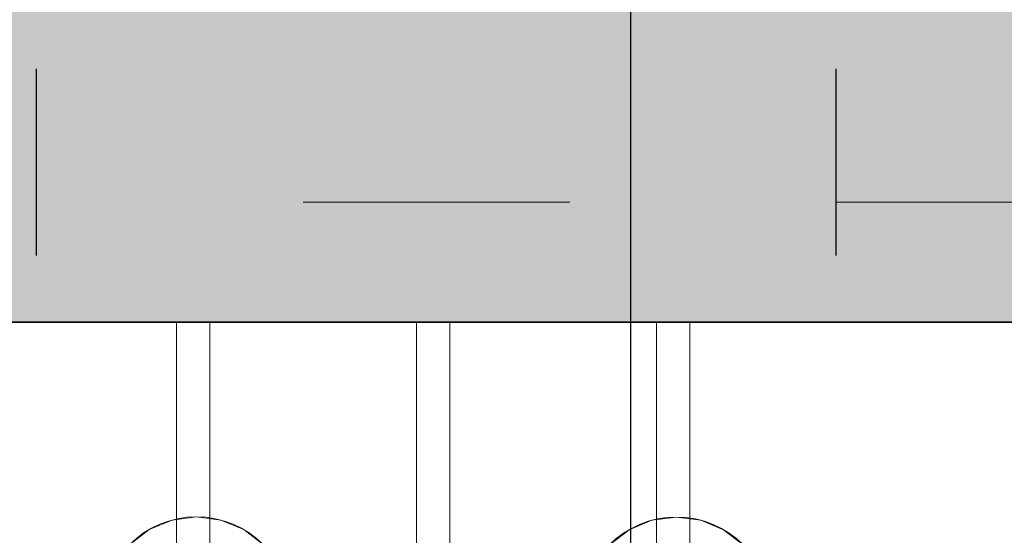
# Model space of a CAD drawing. Units: inches. Extents: x 2696 to 3240, y 1564 to 2310.
# Tile 46 of 76: x 2777.108 to 2786.339, y 2089.203 to 2094.037. Entities that reach past the tile are written whole.
import ezdxf

# ---------------------------------------------------------------- set-up
doc = ezdxf.new("R2010")
doc.units = ezdxf.units.IN
for name, color, linetype, lineweight in [('A-ANNO-DIMS', 3, 'Continuous', 18), ('A-FLOR-FIXT', 8, 'Continuous', 18), ('A-FURN', 251, 'Continuous', 13), ('A-WALL', 7, 'Continuous', 35), ('A-WALL-PATT', 9, 'Continuous', 13)]:
    doc.layers.add(name, color=color, linetype=linetype, lineweight=lineweight)
doc.layers.add('FURNITURE', color=250, linetype='Continuous')
doc.styles.add('TIMES NEW', font='times.ttf')
doc.dimstyles.new('Siddhuu', dxfattribs={"dimtxt": 6, "dimasz": 2.5, "dimexe": 1.25, "dimexo": 0.625, "dimtad": 1, "dimdec": 1, "dimlunit": 4, "dimtxsty": 'TIMES NEW', "dimcen": 2.5, "dimclrd": 256, "dimclre": 1, "dimclrt": 7, "dimadec": 0, "dimazin": 0, "dimtfac": 1, "dimtdec": 1, "dimtmove": 0, "dimatfit": 3, "dimfxl": 1, "dimtolj": 1, "dimlwd": -1, "dimarcsym": 0})

# ---------------------------------------------------------------- blocks, each defined once
blk = doc.blocks.new('A$C1af1f523')
at = {"layer": 'A-FURN'}
for p, q in [((-1.9455, 2.8785), (-1.9455, 2.8785, 0.5)), ((-1.857, 2.6648), (-1.857, 2.6648, 0.5)), ((0, 2.5605), (-4.2116, 2.5605)), ((0, 2.5605, 0.5), (-4.2116, 2.5605, 0.5)), ((-1.8268, 2.4355), (-1.8268, 2.4355, 0.5)), ((0, 2.248), (-4.2116, 2.248)), ((0, 2.248, 0.5), (-4.2116, 2.248, 0.5)), ((-1.857, 2.2061), (-1.857, 2.2061, 0.5)), ((-1.9455, 1.9924), (-1.9455, 1.9924, 0.5)), ((0, 0.3125), (-6.5015, 0.3125)), ((0, 0.3125, 0.5), (-6.5015, 0.3125, 0.5)), ((0, 0), (-6.5015, 0)), ((0, 0, 0.5), (-6.5015, 0, 0.5)), ((-1.9432, -1.6208), (-1.9432, -1.6208, 0.5)), ((-1.8547, -1.8345), (-1.8547, -1.8345, 0.5)), ((0, -1.9388), (-4.2094, -1.9388)), ((0, -1.9388, 0.5), (-4.2094, -1.9388, 0.5)), ((-1.8245, -2.0638), (-1.8245, -2.0638, 0.5)), ((0, -2.2513), (-4.2094, -2.2513)), ((0, -2.2513, 0.5), (-4.2094, -2.2513, 0.5)), ((-1.8547, -2.2931), (-1.8547, -2.2931, 0.5)), ((-1.9432, -2.5068), (-1.9432, -2.5068, 0.5))]:
    blk.add_line(p, q, dxfattribs=at)
for centre in [(-2.7128, 2.4355), (-2.7128, 2.4355, 0.5), (-2.7105, -2.0638), (-2.7105, -2.0638, 0.5)]:
    blk.add_circle(centre, 0.886, dxfattribs=at)
at = {"layer": 'FURNITURE'}
for p, q in [((0, 2.5605), (0, 2.5605, 0.5)), ((0, 2.248), (0, 2.248, 0.5)), ((0, 0.3125), (0, 0.3125, 0.5)), ((0, 0), (0, 0, 0.5)), ((0, -1.9388), (0, -1.9388, 0.5)), ((0, -2.2513), (0, -2.2513, 0.5))]:
    blk.add_line(p, q, dxfattribs=at)
at = {"layer": 'A-FURN'}
mesh = blk.add_polyface(dxfattribs=at)
corners = [(-1.9455, 2.8785, 0.5), (-2.0863, 3.062), (-1.9455, 2.8785), (-2.0863, 3.062, 0.5)]
mesh.append_faces([[corners[k] for k in face] for face in [(2, 1, 0), (3, 0, 1)]], dxfattribs={"vtx1": -1})
mesh = blk.add_polyface(dxfattribs=at)
corners = [(-1.857, 2.6648, 0.5), (-1.9455, 2.8785), (-1.857, 2.6648), (-1.9455, 2.8785, 0.5)]
mesh.append_faces([[corners[k] for k in face] for face in [(2, 1, 0), (3, 0, 1)]], dxfattribs={"vtx1": -1})
mesh = blk.add_polyface(dxfattribs=at)
corners = [(-1.8268, 2.4355, 0.5), (-1.857, 2.6648), (-1.8268, 2.4355), (-1.857, 2.6648, 0.5)]
mesh.append_faces([[corners[k] for k in face] for face in [(2, 1, 0), (3, 0, 1)]], dxfattribs={"vtx1": -1})
mesh = blk.add_polyface(dxfattribs=at)
corners = [(0, 2.5605, 0.5), (-4.2116, 2.5605), (-4.2116, 2.5605, 0.5), (0, 2.5605)]
mesh.append_faces([[corners[k] for k in face] for face in [(2, 1, 0), (3, 0, 1)]], dxfattribs={"vtx1": -1})
mesh = blk.add_polyface(dxfattribs=at)
corners = [(-1.857, 2.2061, 0.5), (-1.8268, 2.4355), (-1.857, 2.2061), (-1.8268, 2.4355, 0.5)]
mesh.append_faces([[corners[k] for k in face] for face in [(2, 1, 0), (3, 0, 1)]], dxfattribs={"vtx1": -1})
mesh = blk.add_polyface(dxfattribs=at)
corners = [(0, 2.248, 0.5), (-4.2116, 2.248), (-4.2116, 2.248, 0.5), (0, 2.248)]
mesh.append_faces([[corners[k] for k in face] for face in [(2, 1, 0), (3, 0, 1)]], dxfattribs={"vtx1": -1})
mesh = blk.add_polyface(dxfattribs=at)
corners = [(-1.9455, 1.9924, 0.5), (-1.857, 2.2061), (-1.9455, 1.9924), (-1.857, 2.2061, 0.5)]
mesh.append_faces([[corners[k] for k in face] for face in [(2, 1, 0), (3, 0, 1)]], dxfattribs={"vtx1": -1})
mesh = blk.add_polyface(dxfattribs=at)
corners = [(-2.0863, 1.8089, 0.5), (-1.9455, 1.9924), (-2.0863, 1.8089), (-1.9455, 1.9924, 0.5)]
mesh.append_faces([[corners[k] for k in face] for face in [(2, 1, 0), (3, 0, 1)]], dxfattribs={"vtx1": -1})
mesh = blk.add_polyface(dxfattribs=at)
corners = [(0, 0.3125, 0.5), (-6.5015, 0.3125), (-6.5015, 0.3125, 0.5), (0, 0.3125)]
mesh.append_faces([[corners[k] for k in face] for face in [(2, 1, 0), (3, 0, 1)]], dxfattribs={"vtx1": -1})
mesh = blk.add_polyface(dxfattribs=at)
corners = [(0, 0, 0.5), (-6.5015, 0), (-6.5015, 0, 0.5), (0, 0)]
mesh.append_faces([[corners[k] for k in face] for face in [(2, 1, 0), (3, 0, 1)]], dxfattribs={"vtx1": -1})
mesh = blk.add_polyface(dxfattribs=at)
corners = [(-1.9432, -1.6208, 0.5), (-2.084, -1.4373), (-1.9432, -1.6208), (-2.084, -1.4373, 0.5)]
mesh.append_faces([[corners[k] for k in face] for face in [(2, 1, 0), (3, 0, 1)]], dxfattribs={"vtx1": -1})
mesh = blk.add_polyface(dxfattribs=at)
corners = [(-1.8547, -1.8345, 0.5), (-1.9432, -1.6208), (-1.8547, -1.8345), (-1.9432, -1.6208, 0.5)]
mesh.append_faces([[corners[k] for k in face] for face in [(2, 1, 0), (3, 0, 1)]], dxfattribs={"vtx1": -1})
mesh = blk.add_polyface(dxfattribs=at)
corners = [(-1.8245, -2.0638, 0.5), (-1.8547, -1.8345), (-1.8245, -2.0638), (-1.8547, -1.8345, 0.5)]
mesh.append_faces([[corners[k] for k in face] for face in [(2, 1, 0), (3, 0, 1)]], dxfattribs={"vtx1": -1})
mesh = blk.add_polyface(dxfattribs=at)
corners = [(0, -1.9388, 0.5), (-4.2094, -1.9388), (-4.2094, -1.9388, 0.5), (0, -1.9388)]
mesh.append_faces([[corners[k] for k in face] for face in [(2, 1, 0), (3, 0, 1)]], dxfattribs={"vtx1": -1})
mesh = blk.add_polyface(dxfattribs=at)
corners = [(-1.8547, -2.2931, 0.5), (-1.8245, -2.0638), (-1.8547, -2.2931), (-1.8245, -2.0638, 0.5)]
mesh.append_faces([[corners[k] for k in face] for face in [(2, 1, 0), (3, 0, 1)]], dxfattribs={"vtx1": -1})
mesh = blk.add_polyface(dxfattribs=at)
corners = [(0, -2.2513, 0.5), (-4.2094, -2.2513), (-4.2094, -2.2513, 0.5), (0, -2.2513)]
mesh.append_faces([[corners[k] for k in face] for face in [(2, 1, 0), (3, 0, 1)]], dxfattribs={"vtx1": -1})
mesh = blk.add_polyface(dxfattribs=at)
corners = [(-1.9432, -2.5068, 0.5), (-1.8547, -2.2931), (-1.9432, -2.5068), (-1.8547, -2.2931, 0.5)]
mesh.append_faces([[corners[k] for k in face] for face in [(2, 1, 0), (3, 0, 1)]], dxfattribs={"vtx1": -1})
mesh = blk.add_polyface(dxfattribs=at)
corners = [(-2.084, -2.6903, 0.5), (-1.9432, -2.5068), (-2.084, -2.6903), (-1.9432, -2.5068, 0.5)]
mesh.append_faces([[corners[k] for k in face] for face in [(2, 1, 0), (3, 0, 1)]], dxfattribs={"vtx1": -1})
blk = doc.blocks.new('*D40')
at = {"layer": 'A-ANNO-DIMS', "color": 1, "lineweight": -2, "transparency": 16777216}
for p, q in [((2777.2662, 2091.8261), (2777.2662, 2093.5758)), ((2784.7641, 2091.8261), (2784.7641, 2093.5758))]:
    blk.add_line(p, q, dxfattribs=at)
at = {"layer": 'A-ANNO-DIMS', "transparency": 16777216}
for p, q in [((2779.7662, 2092.3258), (2782.2641, 2092.3258)), ((2784.7641, 2092.3258), (2902.4579, 2092.3258))]:
    blk.add_line(p, q, dxfattribs=at)
for points in [[(2779.7662, 2092.7424), (2779.7662, 2091.9091), (2777.2662, 2092.3258)], [(2782.2641, 2092.7424), (2782.2641, 2091.9091), (2784.7641, 2092.3258)]]:
    blk.add_solid(points, dxfattribs=at)
at = {"layer": 'Defpoints', "color": 0, "transparency": 16777216}
for p in [(2784.7641, 2092.3258), (2777.2662, 2091.2011), (2784.7641, 2091.2011)]:
    blk.add_point(p, dxfattribs=at)
at = {"layer": 'A-ANNO-DIMS', "color": 7, "transparency": 16777216, "insert": (2844.861, 2096.0935), "char_height": 6, "attachment_point": 5, "style": 'TIMES NEW'}
blk.add_mtext('\\A1;BATH FITTING 0\'-7 1/2" TYP.', dxfattribs=at)
blk = doc.blocks.new('*D41')
at = {"layer": 'A-ANNO-DIMS', "transparency": 16777216}
for p, q in [((2776.1416, 2091.2011), (2776.1416, 2145.7283)), ((2776.1416, 2087.1996), (2776.1416, 2088.7011))]:
    blk.add_line(p, q, dxfattribs=at)
at = {"layer": 'A-ANNO-DIMS', "color": 1, "lineweight": -2, "transparency": 16777216}
for p, q in [((2776.6412, 2091.2011), (2774.8916, 2091.2011)), ((2776.6412, 2084.6996), (2774.8916, 2084.6996))]:
    blk.add_line(p, q, dxfattribs=at)
at = {"layer": 'A-ANNO-DIMS', "transparency": 16777216}
for points in [[(2775.7249, 2088.7011), (2776.5582, 2088.7011), (2776.1416, 2091.2011)], [(2775.7249, 2087.1996), (2776.5582, 2087.1996), (2776.1416, 2084.6996)]]:
    blk.add_solid(points, dxfattribs=at)
at = {"layer": 'Defpoints', "color": 0, "transparency": 16777216}
for p in [(2776.1416, 2091.2011), (2777.2662, 2091.2011), (2777.2662, 2084.6996)]:
    blk.add_point(p, dxfattribs=at)
at = {"layer": 'A-ANNO-DIMS', "color": 7, "transparency": 16777216, "insert": (2772.3803, 2119.7147), "char_height": 6, "attachment_point": 5, "rotation": 90, "style": 'TIMES NEW'}
blk.add_mtext('\\A1;0\'-6 1/2" TYP.', dxfattribs=at)
blk = doc.blocks.new('*D62')
at = {"layer": 'A-ANNO-DIMS', "color": 1, "lineweight": -2, "transparency": 16777216}
for p, q in [((2965.0838, 2140.7011), (2709.3614, 2140.7011)), ((2965.0838, 2063.5906), (2709.3614, 2063.5906))]:
    blk.add_line(p, q, dxfattribs=at)
at = {"layer": 'A-ANNO-DIMS', "transparency": 16777216}
blk.add_line((2710.6114, 2066.0906), (2710.6114, 2138.2011), dxfattribs=at)
for points in [[(2710.1947, 2138.2011), (2711.0281, 2138.2011), (2710.6114, 2140.7011)], [(2710.1947, 2066.0906), (2711.0281, 2066.0906), (2710.6114, 2063.5906)]]:
    blk.add_solid(points, dxfattribs=at)
at = {"layer": 'Defpoints', "color": 0, "transparency": 16777216}
for p in [(2710.6114, 2140.7011), (2965.7088, 2140.7011), (2965.7088, 2063.5906)]:
    blk.add_point(p, dxfattribs=at)
at = {"layer": 'A-ANNO-DIMS', "color": 7, "transparency": 16777216, "insert": (2706.9345, 2102.1459), "char_height": 6, "attachment_point": 5, "rotation": 90, "style": 'TIMES NEW'}
blk.add_mtext('\\A1;6\'-5"', dxfattribs=at)
blk = doc.blocks.new('*D64')
at = {"layer": 'A-ANNO-DIMS', "color": 1, "lineweight": -2, "transparency": 16777216}
for p, q in [((3073.0838, 2206.7011), (2709.3614, 2206.7011)), ((3068.5838, 1989.2011), (2709.3614, 1989.2011))]:
    blk.add_line(p, q, dxfattribs=at)
at = {"layer": 'A-ANNO-DIMS', "transparency": 16777216}
blk.add_line((2710.6114, 1991.7011), (2710.6114, 2204.2011), dxfattribs=at)
for points in [[(2710.1947, 2204.2011), (2711.0281, 2204.2011), (2710.6114, 2206.7011)], [(2710.1947, 1991.7011), (2711.0281, 1991.7011), (2710.6114, 1989.2011)]]:
    blk.add_solid(points, dxfattribs=at)
at = {"layer": 'Defpoints', "color": 0, "transparency": 16777216}
for p in [(2710.6114, 2206.7011), (3073.7088, 2206.7011), (3069.2088, 1989.2011)]:
    blk.add_point(p, dxfattribs=at)
at = {"layer": 'A-ANNO-DIMS', "color": 7, "transparency": 16777216, "insert": (2706.8501, 2097.9511), "char_height": 6, "attachment_point": 5, "rotation": 90, "style": 'TIMES NEW'}
blk.add_mtext('\\A1;18\'-1 1/2"', dxfattribs=at)
blk = doc.blocks.new('*D66')
at = {"layer": 'A-ANNO-DIMS', "color": 1, "lineweight": -2, "transparency": 16777216}
for p, q in [((3077.5838, 2122.7011), (2709.3614, 2122.7011)), ((3077.5838, 2074.7011), (2709.3614, 2074.7011))]:
    blk.add_line(p, q, dxfattribs=at)
at = {"layer": 'A-ANNO-DIMS', "transparency": 16777216}
blk.add_line((2710.6114, 2077.2011), (2710.6114, 2120.2011), dxfattribs=at)
for points in [[(2710.1947, 2120.2011), (2711.0281, 2120.2011), (2710.6114, 2122.7011)], [(2710.1947, 2077.2011), (2711.0281, 2077.2011), (2710.6114, 2074.7011)]]:
    blk.add_solid(points, dxfattribs=at)
at = {"layer": 'Defpoints', "color": 0, "transparency": 16777216}
for p in [(2710.6114, 2122.7011), (3078.2088, 2122.7011), (3078.2088, 2074.7011)]:
    blk.add_point(p, dxfattribs=at)
at = {"layer": 'A-ANNO-DIMS', "color": 7, "transparency": 16777216, "insert": (2706.9345, 2098.7011), "char_height": 6, "attachment_point": 5, "rotation": 90, "style": 'TIMES NEW'}
blk.add_mtext('\\A1;4\'-0"', dxfattribs=at)
blk = doc.blocks.new('*D68')
at = {"layer": 'A-ANNO-DIMS', "color": 1, "lineweight": -2, "transparency": 16777216}
for p, q in [((2745.6114, 2261.5761), (2745.6114, 1568.9511)), ((2782.8338, 2261.5761), (2782.8338, 1568.9511))]:
    blk.add_line(p, q, dxfattribs=at)
at = {"layer": 'A-ANNO-DIMS', "transparency": 16777216}
blk.add_line((2748.1114, 1570.2011), (2780.3338, 1570.2011), dxfattribs=at)
for points in [[(2748.1114, 1570.6178), (2748.1114, 1569.7844), (2745.6114, 1570.2011)], [(2780.3338, 1570.6178), (2780.3338, 1569.7844), (2782.8338, 1570.2011)]]:
    blk.add_solid(points, dxfattribs=at)
at = {"layer": 'Defpoints', "color": 0, "transparency": 16777216}
for p in [(2745.6114, 2262.2011), (2782.8338, 2262.2011), (2782.8338, 1570.2011)]:
    blk.add_point(p, dxfattribs=at)
at = {"layer": 'A-ANNO-DIMS', "color": 7, "transparency": 16777216, "insert": (2764.2226, 1573.878), "char_height": 6, "attachment_point": 5, "style": 'TIMES NEW'}
blk.add_mtext('\\A1;3\'-1"', dxfattribs=at)

msp = doc.modelspace()

# ---------------------------------------------------------------- hatches: boundary and pattern name
at = {"layer": 'A-WALL-PATT', "transparency": 33554556}
h = msp.add_hatch(color=256, dxfattribs=at)
h.dxf.hatch_style = 1
h.paths.add_polyline_path([(2879.1114, 2253.2011), (2905.9101, 2253.2011), (2905.9101, 2262.2011), (2841.889, 2262.2011), (2841.889, 2253.2011), (2870.1114, 2253.2011), (2870.1114, 2176.6011), (2965.7088, 2176.6011), (2965.7088, 2206.7011), (2973.5828, 2206.7011), (2973.5828, 2215.7011), (2965.7088, 2215.7011), (2965.7088, 2262.2011), (2929.9101, 2262.2011), (2929.9101, 2253.2011), (2956.7088, 2253.2011), (2956.7088, 2185.6011), (2879.1114, 2185.6011)])
h.paths.add_polyline_path([(2782.8338, 2262.2011), (2745.6114, 2262.2011), (2745.6114, 2228.7287), (2754.6114, 2228.7287), (2754.6114, 2253.2011), (2782.8338, 2253.2011)])
h.paths.add_polyline_path([(2754.6114, 2136.2011), (2965.7088, 2136.2011), (2965.7088, 2145.2011), (2879.1114, 2145.2011), (2879.1114, 2147.0735), (2877.3397, 2147.0735), (2870.1114, 2147.0735), (2870.1114, 2145.2011), (2754.6114, 2145.2011), (2754.6114, 2169.6735), (2745.6114, 2169.6735), (2745.6114, 2000.2011), (2754.6114, 2000.2011), (2754.6114, 2019.2011), (2849.0828, 2019.2011), (2849.0828, 2023.7011), (2841.2088, 2023.7011), (2841.2088, 2051.8271), (2836.7088, 2051.8271), (2836.7088, 2023.7011), (2754.6114, 2023.7011), (2754.6114, 2091.2011), (2836.7088, 2091.2011), (2836.7088, 2087.8271), (2841.2088, 2087.8271), (2841.2088, 2095.7011), (2754.6114, 2095.7011)])
h.paths.add_polyline_path([(2965.7088, 2136.2011), (2956.7088, 2136.2011), (2956.7088, 2023.7011), (2885.0828, 2023.7011), (2885.0828, 2019.2011), (2956.7088, 2019.2011), (2956.7088, 1950.5751), (2965.7088, 1950.5751), (2965.7088, 1980.2011), (2973.5828, 1980.2011), (2973.5828, 1989.2011), (2965.7088, 1989.2011)])
h.paths.add_polyline_path([(2754.6114, 1906.7011), (2880.2088, 1906.7011), (2884.7088, 1906.7011), (2956.7088, 1906.7011), (2956.7088, 1792.7011), (2944.7088, 1792.7011), (2944.7088, 1783.7011), (2956.7088, 1783.7011), (2956.7088, 1740.2011), (2884.7088, 1740.2011), (2884.7088, 1783.7011), (2896.7088, 1783.7011), (2896.7088, 1792.7011), (2884.7088, 1792.7011), (2884.7088, 1846.7011), (2880.2088, 1846.7011), (2880.2088, 1740.2011), (2754.6114, 1740.2011), (2754.6114, 1777.2011), (2745.6114, 1777.2011), (2745.6114, 1692.7011), (2754.6114, 1692.7011), (2754.6114, 1731.2011), (2956.7088, 1731.2011), (2956.7088, 1723.3271), (2965.7088, 1723.3271), (2965.7088, 1884.2011), (2973.5828, 1884.2011), (2973.5828, 1893.2011), (2965.7088, 1893.2011), (2965.7088, 1914.5751), (2956.7088, 1914.5751), (2956.7088, 1911.2011), (2754.6114, 1911.2011), (2754.6114, 1930.2011), (2745.6114, 1930.2011), (2745.6114, 1817.2011), (2754.6114, 1817.2011), (2754.6114, 1854.2011), (2826.6114, 1854.2011), (2826.6114, 1868.8271), (2822.1114, 1868.8271), (2822.1114, 1858.7011), (2754.6114, 1858.7011)])
h.paths.add_polyline_path([(2965.7088, 1656.2011), (3008.2374, 1656.2011), (3008.2374, 1665.2011), (2965.7088, 1665.2011), (2965.7088, 1693.3271), (2956.7088, 1693.3271), (2956.7088, 1686.2011), (2934.5828, 1686.2011), (2934.5828, 1681.7011), (2956.7088, 1681.7011), (2956.7088, 1614.2011), (2896.7088, 1614.2011), (2896.7088, 1681.7011), (2904.5828, 1681.7011), (2904.5828, 1686.2011), (2892.2088, 1686.2011), (2892.2088, 1614.2011), (2858.4101, 1614.2011), (2858.4101, 1605.2011), (2965.7088, 1605.2011)])
h.paths.add_polyline_path([(2788.4101, 1614.2011), (2754.6114, 1614.2011), (2754.6114, 1652.7011), (2745.6114, 1652.7011), (2745.6114, 1605.2011), (2788.4101, 1605.2011)])
h.paths.add_polyline_path([(3199.6114, 1633.0476), (3190.6114, 1633.0476), (3190.6114, 1614.2011), (3082.6114, 1614.2011), (3082.6114, 1665.2011), (3070.2374, 1665.2011), (3070.2374, 1656.2011), (3078.1114, 1656.2011), (3078.1114, 1605.2011), (3199.6114, 1605.2011)])
h.paths.add_polyline_path([(3199.6114, 1702.0476), (3190.6114, 1702.0476), (3190.6114, 1699.7011), (3106.6114, 1699.7011), (3106.6114, 1747.7011), (3190.6114, 1747.7011), (3190.6114, 1752.2011), (3082.6114, 1752.2011), (3082.6114, 1760.0751), (3078.1114, 1760.0751), (3078.1114, 1747.7011), (3102.1114, 1747.7011), (3102.1114, 1699.7011), (3078.1114, 1699.7011), (3078.1114, 1695.2011), (3190.6114, 1695.2011), (3190.6114, 1676.3546), (3199.6114, 1676.3546)])
h.paths.add_polyline_path([(3199.6114, 1783.2011), (3190.6114, 1783.2011), (3190.6114, 1745.3546), (3199.6114, 1745.3546)])
h.paths.add_polyline_path([(3082.6114, 1884.2011), (3190.6114, 1884.2011), (3190.6114, 1853.2011), (3199.6114, 1853.2011), (3199.6114, 1901.7011), (3190.6114, 1901.7011), (3190.6114, 1893.2011), (3005.5828, 1893.2011), (3005.5828, 1891.2811), (3005.5828, 1884.2011), (3078.1114, 1884.2011), (3078.1114, 1792.0751), (3082.6114, 1792.0751)])
h.paths.add_polyline_path([(3199.6114, 1994.7011), (3190.6114, 1994.7011), (3190.6114, 1989.2011), (3073.7088, 1989.2011), (3073.7088, 2034.2011), (3069.2088, 2034.2011), (3069.2088, 1989.2011), (3005.5828, 1989.2011), (3005.5828, 1980.2011), (3190.6114, 1980.2011), (3190.6114, 1971.7011), (3199.6114, 1971.7011)])
h.paths.add_polyline_path([(3199.6114, 2155.2011), (3190.6114, 2155.2011), (3190.6114, 2064.7011), (3199.6114, 2064.7011)])
h.paths.add_polyline_path([(3190.6114, 2074.7011), (3106.6114, 2074.7011), (3106.6114, 2122.7011), (3190.6114, 2122.7011), (3190.6114, 2127.2011), (3082.7088, 2127.2011), (3082.7088, 2135.0751), (3073.7088, 2135.0751), (3073.7088, 2122.7011), (3102.1114, 2122.7011), (3102.1114, 2074.7011), (3069.2088, 2074.7011), (3069.2088, 2070.2011), (3190.6114, 2070.2011)])
h.paths.add_polyline_path([(3082.7088, 2253.2011), (3190.6114, 2253.2011), (3190.6114, 2225.2011), (3199.6114, 2225.2011), (3199.6114, 2262.2011), (3073.7088, 2262.2011), (3073.7088, 2215.7011), (3035.5828, 2215.7011), (3035.5828, 2206.7011), (3073.7088, 2206.7011), (3073.7088, 2171.0751), (3082.7088, 2171.0751)])

# ---------------------------------------------------------------- linework, layer by layer
at = {"layer": 'A-WALL'}
msp.add_line((2754.6114, 2091.2011), (2836.7088, 2091.2011), dxfattribs=at)

# ---------------------------------------------------------------- block references
at = {"layer": 'A-FLOR-FIXT', "xscale": -1, "rotation": 270}
msp.add_blockref('A$C1af1f523', (2780.829, 2091.2011), dxfattribs=at)

# ---------------------------------------------------------------- dimensions: what is measured, and where the dimension line sits
at = {"layer": 'A-ANNO-DIMS'}
dim = msp.add_linear_dim(base=(2782.8338, 1570.2011), p1=(2745.6114, 2262.2011), p2=(2782.8338, 2262.2011), dimstyle='Siddhuu', override={"dimdec": 1, "dimlfac": 1, "dimrnd": 0, "dimzin": 1, "dimdsep": 46, "dimlunit": 4, "dimfrac": 2}, dxfattribs=at)
dim.commit()
dim.dimension.update_dxf_attribs({"geometry": '*D68', "text_midpoint": (2764.2226, 1573.878)})
for base, p1, p2, picture, middle in [((2710.6114, 2206.7011), (3069.2088, 1989.2011), (3073.7088, 2206.7011), '*D64', (2706.8501, 2097.9511)), ((2710.6114, 2140.7011), (2965.7088, 2063.5906), (2965.7088, 2140.7011), '*D62', (2706.9345, 2102.1459)), ((2710.6114, 2122.7011), (3078.2088, 2074.7011), (3078.2088, 2122.7011), '*D66', (2706.9345, 2098.7011))]:
    dim = msp.add_linear_dim(base=base, p1=p1, p2=p2, angle=90, dimstyle='Siddhuu', override={"dimdec": 1, "dimlfac": 1, "dimrnd": 0, "dimzin": 1, "dimdsep": 46, "dimlunit": 4, "dimfrac": 2}, dxfattribs=at)
    dim.commit()
    dim.dimension.update_dxf_attribs({"geometry": picture, "text_midpoint": middle})
dim = msp.add_linear_dim(base=(2776.1416, 2091.2011), p1=(2777.2662, 2084.6996), p2=(2777.2662, 2091.2011), angle=90, text='<> TYP.', dimstyle='Siddhuu', override={"dimdec": 1, "dimlfac": 1, "dimrnd": 0, "dimzin": 1, "dimdsep": 46, "dimlunit": 4, "dimfrac": 2}, dxfattribs=at)
dim.commit()
dim.dimension.update_dxf_attribs({"geometry": '*D41', "text_midpoint": (2772.3803, 2119.7147)})
dim = msp.add_linear_dim(base=(2784.7641, 2092.3258), p1=(2777.2662, 2091.2011), p2=(2784.7641, 2091.2011), text='BATH FITTING <> TYP.', dimstyle='Siddhuu', override={"dimdec": 1, "dimlfac": 1, "dimrnd": 0, "dimzin": 1, "dimdsep": 46, "dimlunit": 4, "dimfrac": 2}, dxfattribs=at)
dim.commit()
dim.dimension.update_dxf_attribs({"geometry": '*D40', "text_midpoint": (2844.861, 2096.0935)})

doc.saveas('drawing.dxf')
